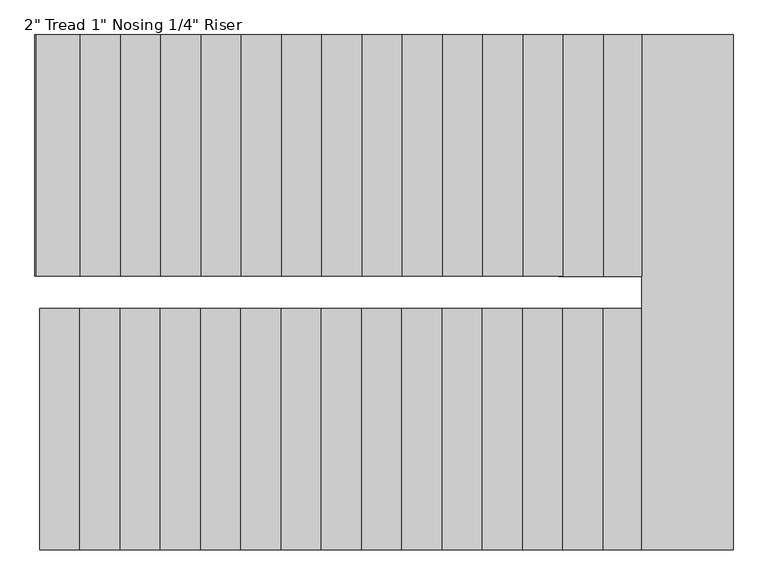
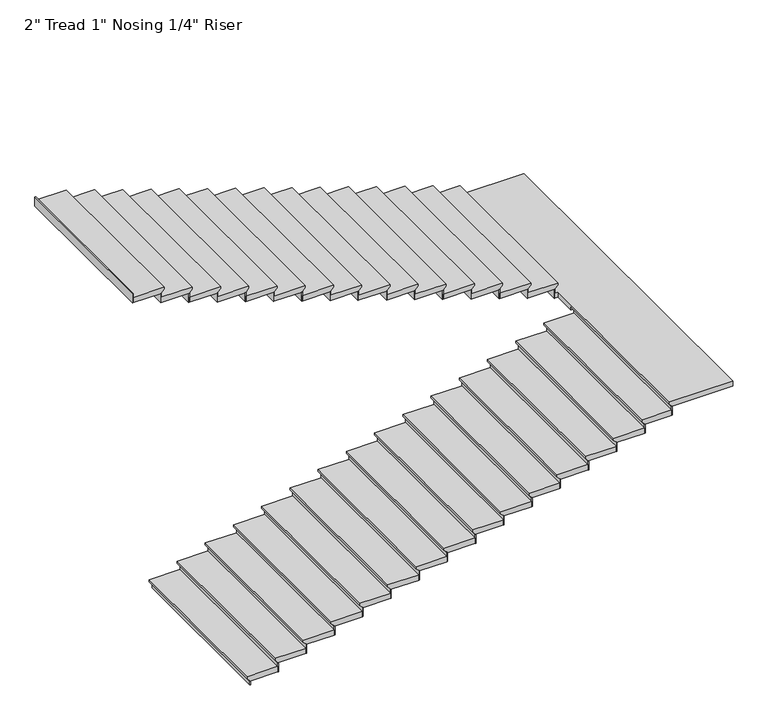
"""IFC4 building model written with IfcOpenShell, lengths in millimetres: stair flight geometry."""

from ifc_helpers import new_model, si_unit, origin, place, context, project, spatial, faceted_brep, source, transform, mapped, element, save


def stair_flight_4f1afc7f(model_context):
    return source(origin(), model_context, "Body", "Brep", [
        faceted_brep([(1449.3932247, -2065.2659014, 3114.675), (1449.3932247, -2065.2659014, 3133.725), (1449.3932247, -541.2659014, 3133.725), (1449.3932247, -541.2659014, 3114.675), (1474.7932247, -2065.2659014, 3089.275), (1474.7932247, -541.2659014, 3089.275), (1726.3621616, -2065.2659014, 3133.725), (1726.3621616, -541.2659014, 3133.725), (1474.7932247, -541.2659014, 3082.925), (1726.3621616, -541.2659014, 3082.925), (1726.3621616, -2065.2659014, 3082.925), (1474.7932247, -2065.2659014, 3082.925)], [[[0, 1, 2, 3]], [[4, 0, 3, 5]], [[2, 1, 6, 7]], [[8, 9, 10, 11]], [[2, 7, 9, 8, 5, 3]], [[8, 11, 4, 5]], [[6, 1, 0, 4, 11, 10]], [[7, 6, 10, 9]]]),
        faceted_brep([(1474.7932247, -2065.2659014, 3082.925), (1474.7932247, -2065.2659014, 3048.0), (1481.1432247, -2065.2659014, 3048.0), (1481.1432247, -2065.2659014, 3082.925), (1474.7932247, -541.2659014, 3082.925), (1481.1432247, -541.2659014, 3082.925), (1481.1432247, -541.2659014, 3048.0), (1474.7932247, -541.2659014, 3048.0)], [[[0, 1, 2, 3]], [[4, 5, 6, 7]], [[1, 0, 4, 7]], [[2, 1, 7, 6]], [[3, 2, 6, 5]], [[0, 3, 5, 4]]]),
        faceted_brep([(1726.3621616, -2065.2659014, 3168.65), (1726.3621616, -2065.2659014, 3082.925), (1732.7121616, -2065.2659014, 3082.925), (1732.7121616, -2065.2659014, 3168.65), (1726.3621616, -541.2659014, 3168.65), (1732.7121616, -541.2659014, 3168.65), (1732.7121616, -541.2659014, 3082.925), (1726.3621616, -541.2659014, 3082.925)], [[[0, 1, 2, 3]], [[4, 5, 6, 7]], [[1, 0, 4, 7]], [[2, 1, 7, 6]], [[3, 2, 6, 5]], [[0, 3, 5, 4]]]),
        faceted_brep([(1700.9621616, -541.2659014, 3219.45), (1700.9621616, -2065.2659014, 3219.45), (1980.3621616, -2065.2659014, 3219.45), (1980.3621616, -541.2659014, 3219.45), (1726.3621616, -541.2659014, 3168.65), (1980.3621616, -541.2659014, 3168.65), (1980.3621616, -2065.2659014, 3168.65), (1726.3621616, -2065.2659014, 3168.65), (1726.3621616, -541.2659014, 3175.0), (1700.9621616, -541.2659014, 3200.4), (1726.3621616, -2065.2659014, 3175.0), (1700.9621616, -2065.2659014, 3200.4)], [[[0, 1, 2, 3]], [[4, 5, 6, 7]], [[0, 3, 5, 4, 8, 9]], [[4, 7, 10, 8]], [[2, 1, 11, 10, 7, 6]], [[3, 2, 6, 5]], [[11, 1, 0, 9]], [[10, 11, 9, 8]]]),
        faceted_brep([(1980.3621616, -2065.2659014, 3254.375), (1980.3621616, -2065.2659014, 3168.65), (1986.7121616, -2065.2659014, 3168.65), (1986.7121616, -2065.2659014, 3254.375), (1980.3621616, -541.2659014, 3254.375), (1986.7121616, -541.2659014, 3254.375), (1986.7121616, -541.2659014, 3168.65), (1980.3621616, -541.2659014, 3168.65)], [[[0, 1, 2, 3]], [[4, 5, 6, 7]], [[1, 0, 4, 7]], [[2, 1, 7, 6]], [[3, 2, 6, 5]], [[0, 3, 5, 4]]]),
        faceted_brep([(1954.9621616, -541.2659014, 3305.175), (1954.9621616, -2065.2659014, 3305.175), (2234.3621616, -2065.2659014, 3305.175), (2234.3621616, -541.2659014, 3305.175), (1980.3621616, -541.2659014, 3254.375), (2234.3621616, -541.2659014, 3254.375), (2234.3621616, -2065.2659014, 3254.375), (1980.3621616, -2065.2659014, 3254.375), (1980.3621616, -541.2659014, 3260.725), (1954.9621616, -541.2659014, 3286.125), (1980.3621616, -2065.2659014, 3260.725), (1954.9621616, -2065.2659014, 3286.125)], [[[0, 1, 2, 3]], [[4, 5, 6, 7]], [[0, 3, 5, 4, 8, 9]], [[4, 7, 10, 8]], [[2, 1, 11, 10, 7, 6]], [[3, 2, 6, 5]], [[11, 1, 0, 9]], [[10, 11, 9, 8]]]),
        faceted_brep([(2234.3621616, -2065.2659014, 3340.1), (2234.3621616, -2065.2659014, 3254.375), (2240.7121616, -2065.2659014, 3254.375), (2240.7121616, -2065.2659014, 3340.1), (2234.3621616, -541.2659014, 3340.1), (2240.7121616, -541.2659014, 3340.1), (2240.7121616, -541.2659014, 3254.375), (2234.3621616, -541.2659014, 3254.375)], [[[0, 1, 2, 3]], [[4, 5, 6, 7]], [[1, 0, 4, 7]], [[2, 1, 7, 6]], [[3, 2, 6, 5]], [[0, 3, 5, 4]]]),
        faceted_brep([(2208.9621616, -541.2659014, 3390.9), (2208.9621616, -2065.2659014, 3390.9), (2488.3621616, -2065.2659014, 3390.9), (2488.3621616, -541.2659014, 3390.9), (2234.3621616, -541.2659014, 3340.1), (2488.3621616, -541.2659014, 3340.1), (2488.3621616, -2065.2659014, 3340.1), (2234.3621616, -2065.2659014, 3340.1), (2234.3621616, -541.2659014, 3346.45), (2208.9621616, -541.2659014, 3371.85), (2234.3621616, -2065.2659014, 3346.45), (2208.9621616, -2065.2659014, 3371.85)], [[[0, 1, 2, 3]], [[4, 5, 6, 7]], [[0, 3, 5, 4, 8, 9]], [[4, 7, 10, 8]], [[2, 1, 11, 10, 7, 6]], [[3, 2, 6, 5]], [[11, 1, 0, 9]], [[10, 11, 9, 8]]]),
        faceted_brep([(2488.3621616, -2065.2659014, 3425.825), (2488.3621616, -2065.2659014, 3340.1), (2494.7121616, -2065.2659014, 3340.1), (2494.7121616, -2065.2659014, 3425.825), (2488.3621616, -541.2659014, 3425.825), (2494.7121616, -541.2659014, 3425.825), (2494.7121616, -541.2659014, 3340.1), (2488.3621616, -541.2659014, 3340.1)], [[[0, 1, 2, 3]], [[4, 5, 6, 7]], [[1, 0, 4, 7]], [[2, 1, 7, 6]], [[3, 2, 6, 5]], [[0, 3, 5, 4]]]),
        faceted_brep([(2462.9621616, -541.2659014, 3476.625), (2462.9621616, -2065.2659014, 3476.625), (2742.3621616, -2065.2659014, 3476.625), (2742.3621616, -541.2659014, 3476.625), (2488.3621616, -541.2659014, 3425.825), (2742.3621616, -541.2659014, 3425.825), (2742.3621616, -2065.2659014, 3425.825), (2488.3621616, -2065.2659014, 3425.825), (2488.3621616, -541.2659014, 3432.175), (2462.9621616, -541.2659014, 3457.575), (2488.3621616, -2065.2659014, 3432.175), (2462.9621616, -2065.2659014, 3457.575)], [[[0, 1, 2, 3]], [[4, 5, 6, 7]], [[0, 3, 5, 4, 8, 9]], [[4, 7, 10, 8]], [[2, 1, 11, 10, 7, 6]], [[3, 2, 6, 5]], [[11, 1, 0, 9]], [[10, 11, 9, 8]]]),
        faceted_brep([(2742.3621616, -2065.2659014, 3511.55), (2742.3621616, -2065.2659014, 3425.825), (2748.7121616, -2065.2659014, 3425.825), (2748.7121616, -2065.2659014, 3511.55), (2742.3621616, -541.2659014, 3511.55), (2748.7121616, -541.2659014, 3511.55), (2748.7121616, -541.2659014, 3425.825), (2742.3621616, -541.2659014, 3425.825)], [[[0, 1, 2, 3]], [[4, 5, 6, 7]], [[1, 0, 4, 7]], [[2, 1, 7, 6]], [[3, 2, 6, 5]], [[0, 3, 5, 4]]]),
        faceted_brep([(2716.9621616, -541.2659014, 3562.35), (2716.9621616, -2065.2659014, 3562.35), (2996.3621616, -2065.2659014, 3562.35), (2996.3621616, -541.2659014, 3562.35), (2742.3621616, -541.2659014, 3511.55), (2996.3621616, -541.2659014, 3511.55), (2996.3621616, -2065.2659014, 3511.55), (2742.3621616, -2065.2659014, 3511.55), (2742.3621616, -541.2659014, 3517.9), (2716.9621616, -541.2659014, 3543.3), (2742.3621616, -2065.2659014, 3517.9), (2716.9621616, -2065.2659014, 3543.3)], [[[0, 1, 2, 3]], [[4, 5, 6, 7]], [[0, 3, 5, 4, 8, 9]], [[4, 7, 10, 8]], [[2, 1, 11, 10, 7, 6]], [[3, 2, 6, 5]], [[11, 1, 0, 9]], [[10, 11, 9, 8]]]),
        faceted_brep([(2996.3621616, -2065.2659014, 3597.275), (2996.3621616, -2065.2659014, 3511.55), (3002.7121616, -2065.2659014, 3511.55), (3002.7121616, -2065.2659014, 3597.275), (2996.3621616, -541.2659014, 3597.275), (3002.7121616, -541.2659014, 3597.275), (3002.7121616, -541.2659014, 3511.55), (2996.3621616, -541.2659014, 3511.55)], [[[0, 1, 2, 3]], [[4, 5, 6, 7]], [[1, 0, 4, 7]], [[2, 1, 7, 6]], [[3, 2, 6, 5]], [[0, 3, 5, 4]]]),
        faceted_brep([(2970.9621616, -541.2659014, 3648.075), (2970.9621616, -2065.2659014, 3648.075), (3250.3621616, -2065.2659014, 3648.075), (3250.3621616, -541.2659014, 3648.075), (2996.3621616, -541.2659014, 3597.275), (3250.3621616, -541.2659014, 3597.275), (3250.3621616, -2065.2659014, 3597.275), (2996.3621616, -2065.2659014, 3597.275), (2996.3621616, -541.2659014, 3603.625), (2970.9621616, -541.2659014, 3629.025), (2996.3621616, -2065.2659014, 3603.625), (2970.9621616, -2065.2659014, 3629.025)], [[[0, 1, 2, 3]], [[4, 5, 6, 7]], [[0, 3, 5, 4, 8, 9]], [[4, 7, 10, 8]], [[2, 1, 11, 10, 7, 6]], [[3, 2, 6, 5]], [[11, 1, 0, 9]], [[10, 11, 9, 8]]]),
        faceted_brep([(3250.3621616, -2065.2659014, 3683.0), (3250.3621616, -2065.2659014, 3597.275), (3256.7121616, -2065.2659014, 3597.275), (3256.7121616, -2065.2659014, 3683.0), (3250.3621616, -541.2659014, 3683.0), (3256.7121616, -541.2659014, 3683.0), (3256.7121616, -541.2659014, 3597.275), (3250.3621616, -541.2659014, 3597.275)], [[[0, 1, 2, 3]], [[4, 5, 6, 7]], [[1, 0, 4, 7]], [[2, 1, 7, 6]], [[3, 2, 6, 5]], [[0, 3, 5, 4]]]),
        faceted_brep([(3224.9621616, -541.2659014, 3733.8), (3224.9621616, -2065.2659014, 3733.8), (3504.3621616, -2065.2659014, 3733.8), (3504.3621616, -541.2659014, 3733.8), (3250.3621616, -541.2659014, 3683.0), (3504.3621616, -541.2659014, 3683.0), (3504.3621616, -2065.2659014, 3683.0), (3250.3621616, -2065.2659014, 3683.0), (3250.3621616, -541.2659014, 3689.35), (3224.9621616, -541.2659014, 3714.75), (3250.3621616, -2065.2659014, 3689.35), (3224.9621616, -2065.2659014, 3714.75)], [[[0, 1, 2, 3]], [[4, 5, 6, 7]], [[0, 3, 5, 4, 8, 9]], [[4, 7, 10, 8]], [[2, 1, 11, 10, 7, 6]], [[3, 2, 6, 5]], [[11, 1, 0, 9]], [[10, 11, 9, 8]]]),
        faceted_brep([(3504.3621616, -2065.2659014, 3768.725), (3504.3621616, -2065.2659014, 3683.0), (3510.7121616, -2065.2659014, 3683.0), (3510.7121616, -2065.2659014, 3768.725), (3504.3621616, -541.2659014, 3768.725), (3510.7121616, -541.2659014, 3768.725), (3510.7121616, -541.2659014, 3683.0), (3504.3621616, -541.2659014, 3683.0)], [[[0, 1, 2, 3]], [[4, 5, 6, 7]], [[1, 0, 4, 7]], [[2, 1, 7, 6]], [[3, 2, 6, 5]], [[0, 3, 5, 4]]]),
        faceted_brep([(3478.9621616, -541.2659014, 3819.525), (3478.9621616, -2065.2659014, 3819.525), (3758.3621616, -2065.2659014, 3819.525), (3758.3621616, -541.2659014, 3819.525), (3504.3621616, -541.2659014, 3768.725), (3758.3621616, -541.2659014, 3768.725), (3758.3621616, -2065.2659014, 3768.725), (3504.3621616, -2065.2659014, 3768.725), (3504.3621616, -541.2659014, 3775.075), (3478.9621616, -541.2659014, 3800.475), (3504.3621616, -2065.2659014, 3775.075), (3478.9621616, -2065.2659014, 3800.475)], [[[0, 1, 2, 3]], [[4, 5, 6, 7]], [[0, 3, 5, 4, 8, 9]], [[4, 7, 10, 8]], [[2, 1, 11, 10, 7, 6]], [[3, 2, 6, 5]], [[11, 1, 0, 9]], [[10, 11, 9, 8]]]),
        faceted_brep([(3758.3621616, -2065.2659014, 3854.45), (3758.3621616, -2065.2659014, 3768.725), (3764.7121616, -2065.2659014, 3768.725), (3764.7121616, -2065.2659014, 3854.45), (3758.3621616, -541.2659014, 3854.45), (3764.7121616, -541.2659014, 3854.45), (3764.7121616, -541.2659014, 3768.725), (3758.3621616, -541.2659014, 3768.725)], [[[0, 1, 2, 3]], [[4, 5, 6, 7]], [[1, 0, 4, 7]], [[2, 1, 7, 6]], [[3, 2, 6, 5]], [[0, 3, 5, 4]]]),
        faceted_brep([(3732.9621616, -541.2659014, 3905.25), (3732.9621616, -2065.2659014, 3905.25), (4012.3621616, -2065.2659014, 3905.25), (4012.3621616, -541.2659014, 3905.25), (3758.3621616, -541.2659014, 3854.45), (4012.3621616, -541.2659014, 3854.45), (4012.3621616, -2065.2659014, 3854.45), (3758.3621616, -2065.2659014, 3854.45), (3758.3621616, -541.2659014, 3860.8), (3732.9621616, -541.2659014, 3886.2), (3758.3621616, -2065.2659014, 3860.8), (3732.9621616, -2065.2659014, 3886.2)], [[[0, 1, 2, 3]], [[4, 5, 6, 7]], [[0, 3, 5, 4, 8, 9]], [[4, 7, 10, 8]], [[2, 1, 11, 10, 7, 6]], [[3, 2, 6, 5]], [[11, 1, 0, 9]], [[10, 11, 9, 8]]]),
        faceted_brep([(4012.3621616, -2065.2659014, 3940.175), (4012.3621616, -2065.2659014, 3854.45), (4018.7121616, -2065.2659014, 3854.45), (4018.7121616, -2065.2659014, 3940.175), (4012.3621616, -541.2659014, 3940.175), (4018.7121616, -541.2659014, 3940.175), (4018.7121616, -541.2659014, 3854.45), (4012.3621616, -541.2659014, 3854.45)], [[[0, 1, 2, 3]], [[4, 5, 6, 7]], [[1, 0, 4, 7]], [[2, 1, 7, 6]], [[3, 2, 6, 5]], [[0, 3, 5, 4]]]),
        faceted_brep([(3986.9621616, -541.2659014, 3990.975), (3986.9621616, -2065.2659014, 3990.975), (4266.3621616, -2065.2659014, 3990.975), (4266.3621616, -541.2659014, 3990.975), (4012.3621616, -541.2659014, 3940.175), (4266.3621616, -541.2659014, 3940.175), (4266.3621616, -2065.2659014, 3940.175), (4012.3621616, -2065.2659014, 3940.175), (4012.3621616, -541.2659014, 3946.525), (3986.9621616, -541.2659014, 3971.925), (4012.3621616, -2065.2659014, 3946.525), (3986.9621616, -2065.2659014, 3971.925)], [[[0, 1, 2, 3]], [[4, 5, 6, 7]], [[0, 3, 5, 4, 8, 9]], [[4, 7, 10, 8]], [[2, 1, 11, 10, 7, 6]], [[3, 2, 6, 5]], [[11, 1, 0, 9]], [[10, 11, 9, 8]]]),
        faceted_brep([(4266.3621616, -2065.2659014, 4025.9), (4266.3621616, -2065.2659014, 3940.175), (4272.7121616, -2065.2659014, 3940.175), (4272.7121616, -2065.2659014, 4025.9), (4266.3621616, -541.2659014, 4025.9), (4272.7121616, -541.2659014, 4025.9), (4272.7121616, -541.2659014, 3940.175), (4266.3621616, -541.2659014, 3940.175)], [[[0, 1, 2, 3]], [[4, 5, 6, 7]], [[1, 0, 4, 7]], [[2, 1, 7, 6]], [[3, 2, 6, 5]], [[0, 3, 5, 4]]]),
        faceted_brep([(4240.9621616, -541.2659014, 4076.7), (4240.9621616, -2065.2659014, 4076.7), (4520.3621616, -2065.2659014, 4076.7), (4520.3621616, -541.2659014, 4076.7), (4266.3621616, -541.2659014, 4025.9), (4520.3621616, -541.2659014, 4025.9), (4520.3621616, -2065.2659014, 4025.9), (4266.3621616, -2065.2659014, 4025.9), (4266.3621616, -541.2659014, 4032.25), (4240.9621616, -541.2659014, 4057.65), (4266.3621616, -2065.2659014, 4032.25), (4240.9621616, -2065.2659014, 4057.65)], [[[0, 1, 2, 3]], [[4, 5, 6, 7]], [[0, 3, 5, 4, 8, 9]], [[4, 7, 10, 8]], [[2, 1, 11, 10, 7, 6]], [[3, 2, 6, 5]], [[11, 1, 0, 9]], [[10, 11, 9, 8]]]),
        faceted_brep([(4520.3621616, -2065.2659014, 4111.625), (4520.3621616, -2065.2659014, 4025.9), (4526.7121616, -2065.2659014, 4025.9), (4526.7121616, -2065.2659014, 4111.625), (4520.3621616, -541.2659014, 4111.625), (4526.7121616, -541.2659014, 4111.625), (4526.7121616, -541.2659014, 4025.9), (4520.3621616, -541.2659014, 4025.9)], [[[0, 1, 2, 3]], [[4, 5, 6, 7]], [[1, 0, 4, 7]], [[2, 1, 7, 6]], [[3, 2, 6, 5]], [[0, 3, 5, 4]]]),
        faceted_brep([(4494.9621616, -541.2659014, 4162.425), (4494.9621616, -2065.2659014, 4162.425), (4774.3621616, -2065.2659014, 4162.425), (4774.3621616, -541.2659014, 4162.425), (4520.3621616, -541.2659014, 4111.625), (4774.3621616, -541.2659014, 4111.625), (4774.3621616, -2065.2659014, 4111.625), (4520.3621616, -2065.2659014, 4111.625), (4520.3621616, -541.2659014, 4117.975), (4494.9621616, -541.2659014, 4143.375), (4520.3621616, -2065.2659014, 4117.975), (4494.9621616, -2065.2659014, 4143.375)], [[[0, 1, 2, 3]], [[4, 5, 6, 7]], [[0, 3, 5, 4, 8, 9]], [[4, 7, 10, 8]], [[2, 1, 11, 10, 7, 6]], [[3, 2, 6, 5]], [[11, 1, 0, 9]], [[10, 11, 9, 8]]]),
        faceted_brep([(4774.3621616, -2065.2659014, 4197.35), (4774.3621616, -2065.2659014, 4111.625), (4780.7121616, -2065.2659014, 4111.625), (4780.7121616, -2065.2659014, 4197.35), (4774.3621616, -541.2659014, 4197.35), (4780.7121616, -541.2659014, 4197.35), (4780.7121616, -541.2659014, 4111.625), (4774.3621616, -541.2659014, 4111.625)], [[[0, 1, 2, 3]], [[4, 5, 6, 7]], [[1, 0, 4, 7]], [[2, 1, 7, 6]], [[3, 2, 6, 5]], [[0, 3, 5, 4]]]),
        faceted_brep([(4748.9621616, -541.2659014, 4248.15), (4748.9621616, -2065.2659014, 4248.15), (5028.3621616, -2065.2659014, 4248.15), (5028.3621616, -541.2659014, 4248.15), (4774.3621616, -541.2659014, 4197.35), (5028.3621616, -541.2659014, 4197.35), (5028.3621616, -2065.2659014, 4197.35), (4774.3621616, -2065.2659014, 4197.35), (4774.3621616, -541.2659014, 4203.7), (4748.9621616, -541.2659014, 4229.1), (4774.3621616, -2065.2659014, 4203.7), (4748.9621616, -2065.2659014, 4229.1)], [[[0, 1, 2, 3]], [[4, 5, 6, 7]], [[0, 3, 5, 4, 8, 9]], [[4, 7, 10, 8]], [[2, 1, 11, 10, 7, 6]], [[3, 2, 6, 5]], [[11, 1, 0, 9]], [[10, 11, 9, 8]]]),
        faceted_brep([(5028.3621616, -2065.2659014, 4283.075), (5028.3621616, -2065.2659014, 4197.35), (5034.7121616, -2065.2659014, 4197.35), (5034.7121616, -2065.2659014, 4283.075), (5028.3621616, -541.2659014, 4283.075), (5034.7121616, -541.2659014, 4283.075), (5034.7121616, -541.2659014, 4197.35), (5028.3621616, -541.2659014, 4197.35)], [[[0, 1, 2, 3]], [[4, 5, 6, 7]], [[1, 0, 4, 7]], [[2, 1, 7, 6]], [[3, 2, 6, 5]], [[0, 3, 5, 4]]]),
        faceted_brep([(5002.9621616, -541.2659014, 4333.875), (5002.9621616, -2065.2659014, 4333.875), (5272.0669505, -2065.2659014, 4333.875), (5272.0669505, -541.2659014, 4333.875), (5028.3621616, -541.2659014, 4283.075), (5272.0669505, -541.2659014, 4283.075), (5272.0669505, -2065.2659014, 4283.075), (5028.3621616, -2065.2659014, 4283.075), (5028.3621616, -541.2659014, 4289.425), (5002.9621616, -541.2659014, 4314.825), (5028.3621616, -2065.2659014, 4289.425), (5002.9621616, -2065.2659014, 4314.825)], [[[0, 1, 2, 3]], [[4, 5, 6, 7]], [[0, 3, 5, 4, 8, 9]], [[4, 7, 10, 8]], [[2, 1, 11, 10, 7, 6]], [[3, 2, 6, 5]], [[11, 1, 0, 9]], [[10, 11, 9, 8]]]),
        faceted_brep([(5272.0669505, -2065.2659014, 4368.8), (5272.0669505, -2065.2659014, 4283.075), (5278.4169505, -2065.2659014, 4283.075), (5278.4169505, -2065.2659014, 4368.8), (5272.0669505, -541.2659014, 4368.8), (5278.4169505, -541.2659014, 4368.8), (5278.4169505, -541.2659014, 4283.075), (5272.0669505, -541.2659014, 4283.075)], [[[0, 1, 2, 3]], [[4, 5, 6, 7]], [[1, 0, 4, 7]], [[2, 1, 7, 6]], [[3, 2, 6, 5]], [[0, 3, 5, 4]]]),
        faceted_brep([(5221.2669505, -337.9910016, 4419.6), (5246.6669505, -337.9910016, 4419.6), (5246.6669505, -2065.2659014, 4419.6), (5822.2548051, -2065.2659014, 4419.6), (5822.2548051, 1185.9340986, 4419.6), (5221.2669505, 1185.9340986, 4419.6), (5246.6669505, -337.9910016, 4368.8), (5221.2669505, -337.9910016, 4368.8), (5221.2669505, 1185.9340986, 4368.8), (5822.2548051, 1185.9340986, 4368.8), (5822.2548051, -2065.2659014, 4368.8), (5272.0669505, -2065.2659014, 4368.8), (5272.0669505, -541.2659014, 4368.8), (5246.6669505, -541.2659014, 4368.8), (5246.6669505, -541.2659014, 4400.55), (5246.6669505, -2065.2659014, 4400.55), (5272.0669505, -541.2659014, 4375.15), (5272.0669505, -2065.2659014, 4375.15)], [[[0, 1, 2, 3, 4, 5]], [[6, 7, 8, 9, 10, 11, 12, 13]], [[1, 0, 7, 6]], [[2, 1, 6, 13, 14, 15]], [[13, 12, 16, 14]], [[12, 11, 17, 16]], [[3, 2, 15, 17, 11, 10]], [[4, 3, 10, 9]], [[5, 4, 9, 8]], [[0, 5, 8, 7]], [[17, 15, 14, 16]]]),
        faceted_brep([(5221.2669505, 1185.9340986, 4454.525), (5221.2669505, 1185.9340986, 4368.8), (5214.9169505, 1185.9340986, 4368.8), (5214.9169505, 1185.9340986, 4454.525), (5221.2669505, -337.9910016, 4454.525), (5214.9169505, -337.9910016, 4454.525), (5214.9169505, -337.9910016, 4368.8), (5221.2669505, -337.9910016, 4368.8)], [[[0, 1, 2, 3]], [[4, 5, 6, 7]], [[1, 0, 4, 7]], [[2, 1, 7, 6]], [[3, 2, 6, 5]], [[0, 3, 5, 4]]]),
        faceted_brep([(5246.6669505, -337.9910016, 4505.325), (5246.6669505, 1185.9340986, 4505.325), (4977.5621616, 1185.9340986, 4505.325), (4977.5621616, -337.9910016, 4505.325), (5221.2669505, -337.9910016, 4454.525), (4977.5621616, -337.9910016, 4454.525), (4977.5621616, 1185.9340986, 4454.525), (5221.2669505, 1185.9340986, 4454.525), (5221.2669505, -337.9910016, 4460.875), (5246.6669505, -337.9910016, 4486.275), (5221.2669505, 1185.9340986, 4460.875), (5246.6669505, 1185.9340986, 4486.275)], [[[0, 1, 2, 3]], [[4, 5, 6, 7]], [[0, 3, 5, 4, 8, 9]], [[4, 7, 10, 8]], [[2, 1, 11, 10, 7, 6]], [[3, 2, 6, 5]], [[11, 1, 0, 9]], [[10, 11, 9, 8]]]),
        faceted_brep([(4977.5621616, 1185.9340986, 4540.25), (4977.5621616, 1185.9340986, 4454.525), (4971.2121616, 1185.9340986, 4454.525), (4971.2121616, 1185.9340986, 4540.25), (4977.5621616, -337.9910016, 4540.25), (4971.2121616, -337.9910016, 4540.25), (4971.2121616, -337.9910016, 4454.525), (4977.5621616, -337.9910016, 4454.525)], [[[0, 1, 2, 3]], [[4, 5, 6, 7]], [[1, 0, 4, 7]], [[2, 1, 7, 6]], [[3, 2, 6, 5]], [[0, 3, 5, 4]]]),
        faceted_brep([(5002.9621616, -337.9910016, 4591.05), (5002.9621616, 1185.9340986, 4591.05), (4723.5621616, 1185.9340986, 4591.05), (4723.5621616, -337.9910016, 4591.05), (4977.5621616, -337.9910016, 4540.25), (4723.5621616, -337.9910016, 4540.25), (4723.5621616, 1185.9340986, 4540.25), (4977.5621616, 1185.9340986, 4540.25), (4977.5621616, -337.9910016, 4546.6), (5002.9621616, -337.9910016, 4572.0), (4977.5621616, 1185.9340986, 4546.6), (5002.9621616, 1185.9340986, 4572.0)], [[[0, 1, 2, 3]], [[4, 5, 6, 7]], [[0, 3, 5, 4, 8, 9]], [[4, 7, 10, 8]], [[2, 1, 11, 10, 7, 6]], [[3, 2, 6, 5]], [[11, 1, 0, 9]], [[10, 11, 9, 8]]]),
        faceted_brep([(4723.5621616, 1185.9340986, 4625.975), (4723.5621616, 1185.9340986, 4540.25), (4717.2121616, 1185.9340986, 4540.25), (4717.2121616, 1185.9340986, 4625.975), (4723.5621616, -337.9910016, 4625.975), (4717.2121616, -337.9910016, 4625.975), (4717.2121616, -337.9910016, 4540.25), (4723.5621616, -337.9910016, 4540.25)], [[[0, 1, 2, 3]], [[4, 5, 6, 7]], [[1, 0, 4, 7]], [[2, 1, 7, 6]], [[3, 2, 6, 5]], [[0, 3, 5, 4]]]),
        faceted_brep([(4748.9621616, -337.9910016, 4676.775), (4748.9621616, 1185.9340986, 4676.775), (4469.5621616, 1185.9340986, 4676.775), (4469.5621616, -337.9910016, 4676.775), (4723.5621616, -337.9910016, 4625.975), (4469.5621616, -337.9910016, 4625.975), (4469.5621616, 1185.9340986, 4625.975), (4723.5621616, 1185.9340986, 4625.975), (4723.5621616, -337.9910016, 4632.325), (4748.9621616, -337.9910016, 4657.725), (4723.5621616, 1185.9340986, 4632.325), (4748.9621616, 1185.9340986, 4657.725)], [[[0, 1, 2, 3]], [[4, 5, 6, 7]], [[0, 3, 5, 4, 8, 9]], [[4, 7, 10, 8]], [[2, 1, 11, 10, 7, 6]], [[3, 2, 6, 5]], [[11, 1, 0, 9]], [[10, 11, 9, 8]]]),
        faceted_brep([(4469.5621616, 1185.9340986, 4711.7), (4469.5621616, 1185.9340986, 4625.975), (4463.2121616, 1185.9340986, 4625.975), (4463.2121616, 1185.9340986, 4711.7), (4469.5621616, -337.9910016, 4711.7), (4463.2121616, -337.9910016, 4711.7), (4463.2121616, -337.9910016, 4625.975), (4469.5621616, -337.9910016, 4625.975)], [[[0, 1, 2, 3]], [[4, 5, 6, 7]], [[1, 0, 4, 7]], [[2, 1, 7, 6]], [[3, 2, 6, 5]], [[0, 3, 5, 4]]]),
        faceted_brep([(4494.9621616, -337.9910016, 4762.5), (4494.9621616, 1185.9340986, 4762.5), (4215.5621616, 1185.9340986, 4762.5), (4215.5621616, -337.9910016, 4762.5), (4469.5621616, -337.9910016, 4711.7), (4215.5621616, -337.9910016, 4711.7), (4215.5621616, 1185.9340986, 4711.7), (4469.5621616, 1185.9340986, 4711.7), (4469.5621616, -337.9910016, 4718.05), (4494.9621616, -337.9910016, 4743.45), (4469.5621616, 1185.9340986, 4718.05), (4494.9621616, 1185.9340986, 4743.45)], [[[0, 1, 2, 3]], [[4, 5, 6, 7]], [[0, 3, 5, 4, 8, 9]], [[4, 7, 10, 8]], [[2, 1, 11, 10, 7, 6]], [[3, 2, 6, 5]], [[11, 1, 0, 9]], [[10, 11, 9, 8]]]),
        faceted_brep([(4215.5621616, 1185.9340986, 4797.425), (4215.5621616, 1185.9340986, 4711.7), (4209.2121616, 1185.9340986, 4711.7), (4209.2121616, 1185.9340986, 4797.425), (4215.5621616, -337.9910016, 4797.425), (4209.2121616, -337.9910016, 4797.425), (4209.2121616, -337.9910016, 4711.7), (4215.5621616, -337.9910016, 4711.7)], [[[0, 1, 2, 3]], [[4, 5, 6, 7]], [[1, 0, 4, 7]], [[2, 1, 7, 6]], [[3, 2, 6, 5]], [[0, 3, 5, 4]]]),
        faceted_brep([(4240.9621616, -337.9910016, 4848.225), (4240.9621616, 1185.9340986, 4848.225), (3961.5621616, 1185.9340986, 4848.225), (3961.5621616, -337.9910016, 4848.225), (4215.5621616, -337.9910016, 4797.425), (3961.5621616, -337.9910016, 4797.425), (3961.5621616, 1185.9340986, 4797.425), (4215.5621616, 1185.9340986, 4797.425), (4215.5621616, -337.9910016, 4803.775), (4240.9621616, -337.9910016, 4829.175), (4215.5621616, 1185.9340986, 4803.775), (4240.9621616, 1185.9340986, 4829.175)], [[[0, 1, 2, 3]], [[4, 5, 6, 7]], [[0, 3, 5, 4, 8, 9]], [[4, 7, 10, 8]], [[2, 1, 11, 10, 7, 6]], [[3, 2, 6, 5]], [[11, 1, 0, 9]], [[10, 11, 9, 8]]]),
        faceted_brep([(3961.5621616, 1185.9340986, 4883.15), (3961.5621616, 1185.9340986, 4797.425), (3955.2121616, 1185.9340986, 4797.425), (3955.2121616, 1185.9340986, 4883.15), (3961.5621616, -337.9910016, 4883.15), (3955.2121616, -337.9910016, 4883.15), (3955.2121616, -337.9910016, 4797.425), (3961.5621616, -337.9910016, 4797.425)], [[[0, 1, 2, 3]], [[4, 5, 6, 7]], [[1, 0, 4, 7]], [[2, 1, 7, 6]], [[3, 2, 6, 5]], [[0, 3, 5, 4]]]),
        faceted_brep([(3986.9621616, -337.9910016, 4933.95), (3986.9621616, 1185.9340986, 4933.95), (3707.5621616, 1185.9340986, 4933.95), (3707.5621616, -337.9910016, 4933.95), (3961.5621616, -337.9910016, 4883.15), (3707.5621616, -337.9910016, 4883.15), (3707.5621616, 1185.9340986, 4883.15), (3961.5621616, 1185.9340986, 4883.15), (3961.5621616, -337.9910016, 4889.5), (3986.9621616, -337.9910016, 4914.9), (3961.5621616, 1185.9340986, 4889.5), (3986.9621616, 1185.9340986, 4914.9)], [[[0, 1, 2, 3]], [[4, 5, 6, 7]], [[0, 3, 5, 4, 8, 9]], [[4, 7, 10, 8]], [[2, 1, 11, 10, 7, 6]], [[3, 2, 6, 5]], [[11, 1, 0, 9]], [[10, 11, 9, 8]]]),
        faceted_brep([(3707.5621616, 1185.9340986, 4968.875), (3707.5621616, 1185.9340986, 4883.15), (3701.2121616, 1185.9340986, 4883.15), (3701.2121616, 1185.9340986, 4968.875), (3707.5621616, -337.9910016, 4968.875), (3701.2121616, -337.9910016, 4968.875), (3701.2121616, -337.9910016, 4883.15), (3707.5621616, -337.9910016, 4883.15)], [[[0, 1, 2, 3]], [[4, 5, 6, 7]], [[1, 0, 4, 7]], [[2, 1, 7, 6]], [[3, 2, 6, 5]], [[0, 3, 5, 4]]]),
        faceted_brep([(3732.9621616, -337.9910016, 5019.675), (3732.9621616, 1185.9340986, 5019.675), (3453.5621616, 1185.9340986, 5019.675), (3453.5621616, -337.9910016, 5019.675), (3707.5621616, -337.9910016, 4968.875), (3453.5621616, -337.9910016, 4968.875), (3453.5621616, 1185.9340986, 4968.875), (3707.5621616, 1185.9340986, 4968.875), (3707.5621616, -337.9910016, 4975.225), (3732.9621616, -337.9910016, 5000.625), (3707.5621616, 1185.9340986, 4975.225), (3732.9621616, 1185.9340986, 5000.625)], [[[0, 1, 2, 3]], [[4, 5, 6, 7]], [[0, 3, 5, 4, 8, 9]], [[4, 7, 10, 8]], [[2, 1, 11, 10, 7, 6]], [[3, 2, 6, 5]], [[11, 1, 0, 9]], [[10, 11, 9, 8]]]),
        faceted_brep([(3453.5621616, 1185.9340986, 5054.6), (3453.5621616, 1185.9340986, 4968.875), (3447.2121616, 1185.9340986, 4968.875), (3447.2121616, 1185.9340986, 5054.6), (3453.5621616, -337.9910016, 5054.6), (3447.2121616, -337.9910016, 5054.6), (3447.2121616, -337.9910016, 4968.875), (3453.5621616, -337.9910016, 4968.875)], [[[0, 1, 2, 3]], [[4, 5, 6, 7]], [[1, 0, 4, 7]], [[2, 1, 7, 6]], [[3, 2, 6, 5]], [[0, 3, 5, 4]]]),
        faceted_brep([(3478.9621616, -337.9910016, 5105.4), (3478.9621616, 1185.9340986, 5105.4), (3199.5621616, 1185.9340986, 5105.4), (3199.5621616, -337.9910016, 5105.4), (3453.5621616, -337.9910016, 5054.6), (3199.5621616, -337.9910016, 5054.6), (3199.5621616, 1185.9340986, 5054.6), (3453.5621616, 1185.9340986, 5054.6), (3453.5621616, -337.9910016, 5060.95), (3478.9621616, -337.9910016, 5086.35), (3453.5621616, 1185.9340986, 5060.95), (3478.9621616, 1185.9340986, 5086.35)], [[[0, 1, 2, 3]], [[4, 5, 6, 7]], [[0, 3, 5, 4, 8, 9]], [[4, 7, 10, 8]], [[2, 1, 11, 10, 7, 6]], [[3, 2, 6, 5]], [[11, 1, 0, 9]], [[10, 11, 9, 8]]]),
        faceted_brep([(3199.5621616, 1185.9340986, 5140.325), (3199.5621616, 1185.9340986, 5054.6), (3193.2121616, 1185.9340986, 5054.6), (3193.2121616, 1185.9340986, 5140.325), (3199.5621616, -337.9910016, 5140.325), (3193.2121616, -337.9910016, 5140.325), (3193.2121616, -337.9910016, 5054.6), (3199.5621616, -337.9910016, 5054.6)], [[[0, 1, 2, 3]], [[4, 5, 6, 7]], [[1, 0, 4, 7]], [[2, 1, 7, 6]], [[3, 2, 6, 5]], [[0, 3, 5, 4]]]),
        faceted_brep([(3224.9621616, -337.9910016, 5191.125), (3224.9621616, 1185.9340986, 5191.125), (2945.5621616, 1185.9340986, 5191.125), (2945.5621616, -337.9910016, 5191.125), (3199.5621616, -337.9910016, 5140.325), (2945.5621616, -337.9910016, 5140.325), (2945.5621616, 1185.9340986, 5140.325), (3199.5621616, 1185.9340986, 5140.325), (3199.5621616, -337.9910016, 5146.675), (3224.9621616, -337.9910016, 5172.075), (3199.5621616, 1185.9340986, 5146.675), (3224.9621616, 1185.9340986, 5172.075)], [[[0, 1, 2, 3]], [[4, 5, 6, 7]], [[0, 3, 5, 4, 8, 9]], [[4, 7, 10, 8]], [[2, 1, 11, 10, 7, 6]], [[3, 2, 6, 5]], [[11, 1, 0, 9]], [[10, 11, 9, 8]]]),
        faceted_brep([(2945.5621616, 1185.9340986, 5226.05), (2945.5621616, 1185.9340986, 5140.325), (2939.2121616, 1185.9340986, 5140.325), (2939.2121616, 1185.9340986, 5226.05), (2945.5621616, -337.9910016, 5226.05), (2939.2121616, -337.9910016, 5226.05), (2939.2121616, -337.9910016, 5140.325), (2945.5621616, -337.9910016, 5140.325)], [[[0, 1, 2, 3]], [[4, 5, 6, 7]], [[1, 0, 4, 7]], [[2, 1, 7, 6]], [[3, 2, 6, 5]], [[0, 3, 5, 4]]]),
        faceted_brep([(2970.9621616, -337.9910016, 5276.85), (2970.9621616, 1185.9340986, 5276.85), (2691.5621616, 1185.9340986, 5276.85), (2691.5621616, -337.9910016, 5276.85), (2945.5621616, -337.9910016, 5226.05), (2691.5621616, -337.9910016, 5226.05), (2691.5621616, 1185.9340986, 5226.05), (2945.5621616, 1185.9340986, 5226.05), (2945.5621616, -337.9910016, 5232.4), (2970.9621616, -337.9910016, 5257.8), (2945.5621616, 1185.9340986, 5232.4), (2970.9621616, 1185.9340986, 5257.8)], [[[0, 1, 2, 3]], [[4, 5, 6, 7]], [[0, 3, 5, 4, 8, 9]], [[4, 7, 10, 8]], [[2, 1, 11, 10, 7, 6]], [[3, 2, 6, 5]], [[11, 1, 0, 9]], [[10, 11, 9, 8]]]),
        faceted_brep([(2691.5621616, 1185.9340986, 5311.775), (2691.5621616, 1185.9340986, 5226.05), (2685.2121616, 1185.9340986, 5226.05), (2685.2121616, 1185.9340986, 5311.775), (2691.5621616, -337.9910016, 5311.775), (2685.2121616, -337.9910016, 5311.775), (2685.2121616, -337.9910016, 5226.05), (2691.5621616, -337.9910016, 5226.05)], [[[0, 1, 2, 3]], [[4, 5, 6, 7]], [[1, 0, 4, 7]], [[2, 1, 7, 6]], [[3, 2, 6, 5]], [[0, 3, 5, 4]]]),
        faceted_brep([(2716.9621616, -337.9910016, 5362.575), (2716.9621616, 1185.9340986, 5362.575), (2437.5621616, 1185.9340986, 5362.575), (2437.5621616, -337.9910016, 5362.575), (2691.5621616, -337.9910016, 5311.775), (2437.5621616, -337.9910016, 5311.775), (2437.5621616, 1185.9340986, 5311.775), (2691.5621616, 1185.9340986, 5311.775), (2691.5621616, -337.9910016, 5318.125), (2716.9621616, -337.9910016, 5343.525), (2691.5621616, 1185.9340986, 5318.125), (2716.9621616, 1185.9340986, 5343.525)], [[[0, 1, 2, 3]], [[4, 5, 6, 7]], [[0, 3, 5, 4, 8, 9]], [[4, 7, 10, 8]], [[2, 1, 11, 10, 7, 6]], [[3, 2, 6, 5]], [[11, 1, 0, 9]], [[10, 11, 9, 8]]]),
        faceted_brep([(2437.5621616, 1185.9340986, 5397.5), (2437.5621616, 1185.9340986, 5311.775), (2431.2121616, 1185.9340986, 5311.775), (2431.2121616, 1185.9340986, 5397.5), (2437.5621616, -337.9910016, 5397.5), (2431.2121616, -337.9910016, 5397.5), (2431.2121616, -337.9910016, 5311.775), (2437.5621616, -337.9910016, 5311.775)], [[[0, 1, 2, 3]], [[4, 5, 6, 7]], [[1, 0, 4, 7]], [[2, 1, 7, 6]], [[3, 2, 6, 5]], [[0, 3, 5, 4]]]),
        faceted_brep([(2462.9621616, -337.9910016, 5448.3), (2462.9621616, 1185.9340986, 5448.3), (2183.5621616, 1185.9340986, 5448.3), (2183.5621616, -337.9910016, 5448.3), (2437.5621616, -337.9910016, 5397.5), (2183.5621616, -337.9910016, 5397.5), (2183.5621616, 1185.9340986, 5397.5), (2437.5621616, 1185.9340986, 5397.5), (2437.5621616, -337.9910016, 5403.85), (2462.9621616, -337.9910016, 5429.25), (2437.5621616, 1185.9340986, 5403.85), (2462.9621616, 1185.9340986, 5429.25)], [[[0, 1, 2, 3]], [[4, 5, 6, 7]], [[0, 3, 5, 4, 8, 9]], [[4, 7, 10, 8]], [[2, 1, 11, 10, 7, 6]], [[3, 2, 6, 5]], [[11, 1, 0, 9]], [[10, 11, 9, 8]]]),
        faceted_brep([(2183.5621616, 1185.9340986, 5483.225), (2183.5621616, 1185.9340986, 5397.5), (2177.2121616, 1185.9340986, 5397.5), (2177.2121616, 1185.9340986, 5483.225), (2183.5621616, -337.9910016, 5483.225), (2177.2121616, -337.9910016, 5483.225), (2177.2121616, -337.9910016, 5397.5), (2183.5621616, -337.9910016, 5397.5)], [[[0, 1, 2, 3]], [[4, 5, 6, 7]], [[1, 0, 4, 7]], [[2, 1, 7, 6]], [[3, 2, 6, 5]], [[0, 3, 5, 4]]]),
        faceted_brep([(2208.9621616, -337.9910016, 5534.025), (2208.9621616, 1185.9340986, 5534.025), (1929.5621616, 1185.9340986, 5534.025), (1929.5621616, -337.9910016, 5534.025), (2183.5621616, -337.9910016, 5483.225), (1929.5621616, -337.9910016, 5483.225), (1929.5621616, 1185.9340986, 5483.225), (2183.5621616, 1185.9340986, 5483.225), (2183.5621616, -337.9910016, 5489.575), (2208.9621616, -337.9910016, 5514.975), (2183.5621616, 1185.9340986, 5489.575), (2208.9621616, 1185.9340986, 5514.975)], [[[0, 1, 2, 3]], [[4, 5, 6, 7]], [[0, 3, 5, 4, 8, 9]], [[4, 7, 10, 8]], [[2, 1, 11, 10, 7, 6]], [[3, 2, 6, 5]], [[11, 1, 0, 9]], [[10, 11, 9, 8]]]),
        faceted_brep([(1929.5621616, 1185.9340986, 5568.95), (1929.5621616, 1185.9340986, 5483.225), (1923.2121616, 1185.9340986, 5483.225), (1923.2121616, 1185.9340986, 5568.95), (1929.5621616, -337.9910016, 5568.95), (1923.2121616, -337.9910016, 5568.95), (1923.2121616, -337.9910016, 5483.225), (1929.5621616, -337.9910016, 5483.225)], [[[0, 1, 2, 3]], [[4, 5, 6, 7]], [[1, 0, 4, 7]], [[2, 1, 7, 6]], [[3, 2, 6, 5]], [[0, 3, 5, 4]]]),
        faceted_brep([(1954.9621616, -337.9910016, 5619.75), (1954.9621616, 1185.9340986, 5619.75), (1675.5621616, 1185.9340986, 5619.75), (1675.5621616, -337.9910016, 5619.75), (1929.5621616, -337.9910016, 5568.95), (1675.5621616, -337.9910016, 5568.95), (1675.5621616, 1185.9340986, 5568.95), (1929.5621616, 1185.9340986, 5568.95), (1929.5621616, -337.9910016, 5575.3), (1954.9621616, -337.9910016, 5600.7), (1929.5621616, 1185.9340986, 5575.3), (1954.9621616, 1185.9340986, 5600.7)], [[[0, 1, 2, 3]], [[4, 5, 6, 7]], [[0, 3, 5, 4, 8, 9]], [[4, 7, 10, 8]], [[2, 1, 11, 10, 7, 6]], [[3, 2, 6, 5]], [[11, 1, 0, 9]], [[10, 11, 9, 8]]]),
        faceted_brep([(1675.5621616, 1185.9340986, 5654.675), (1675.5621616, 1185.9340986, 5568.95), (1669.2121616, 1185.9340986, 5568.95), (1669.2121616, 1185.9340986, 5654.675), (1675.5621616, -337.9910016, 5654.675), (1669.2121616, -337.9910016, 5654.675), (1669.2121616, -337.9910016, 5568.95), (1675.5621616, -337.9910016, 5568.95)], [[[0, 1, 2, 3]], [[4, 5, 6, 7]], [[1, 0, 4, 7]], [[2, 1, 7, 6]], [[3, 2, 6, 5]], [[0, 3, 5, 4]]]),
        faceted_brep([(1423.9932247, 1185.9340986, 5740.4), (1423.9932247, 1185.9340986, 5654.675), (1417.6432247, 1185.9340986, 5654.675), (1417.6432247, 1185.9340986, 5740.4), (1423.9932247, -337.9910016, 5740.4), (1417.6432247, -337.9910016, 5740.4), (1417.6432247, -337.9910016, 5654.675), (1423.9932247, -337.9910016, 5654.675)], [[[0, 1, 2, 3]], [[4, 5, 6, 7]], [[1, 0, 4, 7]], [[2, 1, 7, 6]], [[3, 2, 6, 5]], [[0, 3, 5, 4]]]),
        faceted_brep([(1700.9621616, -337.9910016, 5705.475), (1700.9621616, 1185.9340986, 5705.475), (1423.9932247, 1185.9340986, 5705.475), (1423.9932247, -337.9910016, 5705.475), (1675.5621616, -337.9910016, 5654.675), (1423.9932247, -337.9910016, 5654.675), (1423.9932247, 1185.9340986, 5654.675), (1675.5621616, 1185.9340986, 5654.675), (1675.5621616, -337.9910016, 5661.025), (1700.9621616, -337.9910016, 5686.425), (1675.5621616, 1185.9340986, 5661.025), (1700.9621616, 1185.9340986, 5686.425)], [[[0, 1, 2, 3]], [[4, 5, 6, 7]], [[0, 3, 5, 4, 8, 9]], [[4, 7, 10, 8]], [[2, 1, 11, 10, 7, 6]], [[3, 2, 6, 5]], [[11, 1, 0, 9]], [[10, 11, 9, 8]]]),
    ])


if __name__ == "__main__":
    model = new_model("IFC4")
    model_context = context("Model", 3, world=origin())
    ifc_project = project(units=[si_unit("LENGTHUNIT", "METRE", prefix="MILLI")], contexts=[model_context])
    site = spatial("IfcSite", under=ifc_project)
    building = spatial("IfcBuilding", under=site)
    placement = place(None, origin())
    stair_flight_shape = stair_flight_4f1afc7f(model_context)
    element("IfcStairFlight", 1, ObjectType="2\" Tread 1\" Nosing 1/4\" Riser", at=placement, inside=building, context=model_context, shape_type="MappedRepresentation", body=[
        mapped(stair_flight_shape, transform((0.0, 0.0, 0.0), x_axis=(1.0, 0.0, 0.0), y_axis=(0.0, 1.0, 0.0), z_axis=(0.0, 0.0, 1.0))),
    ])
    save(model, "model.ifc")
